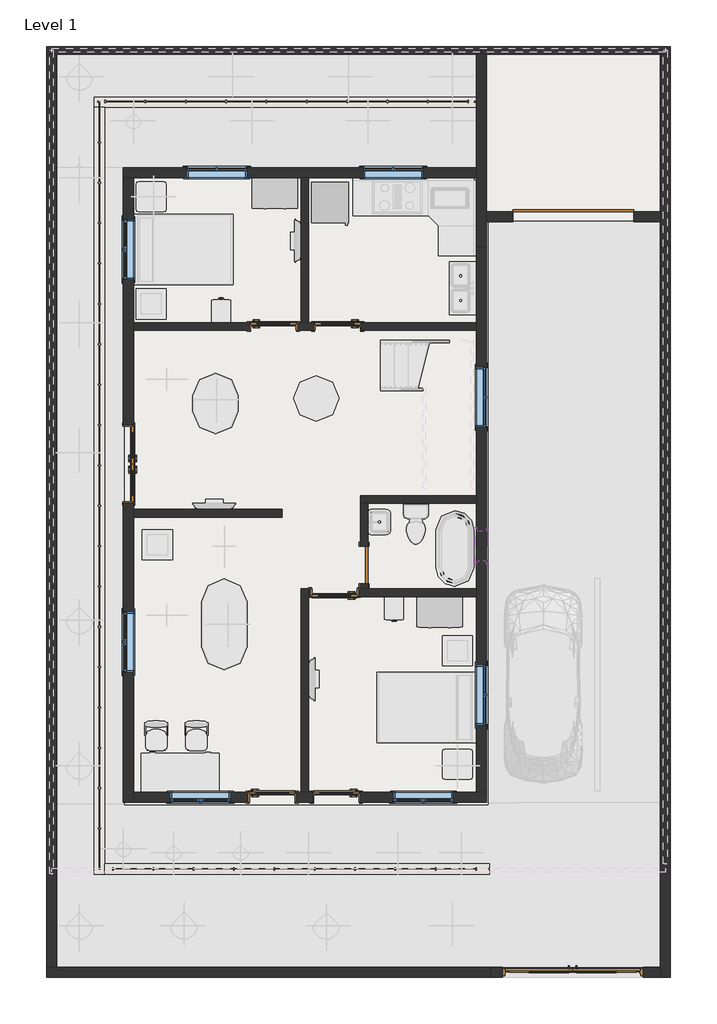
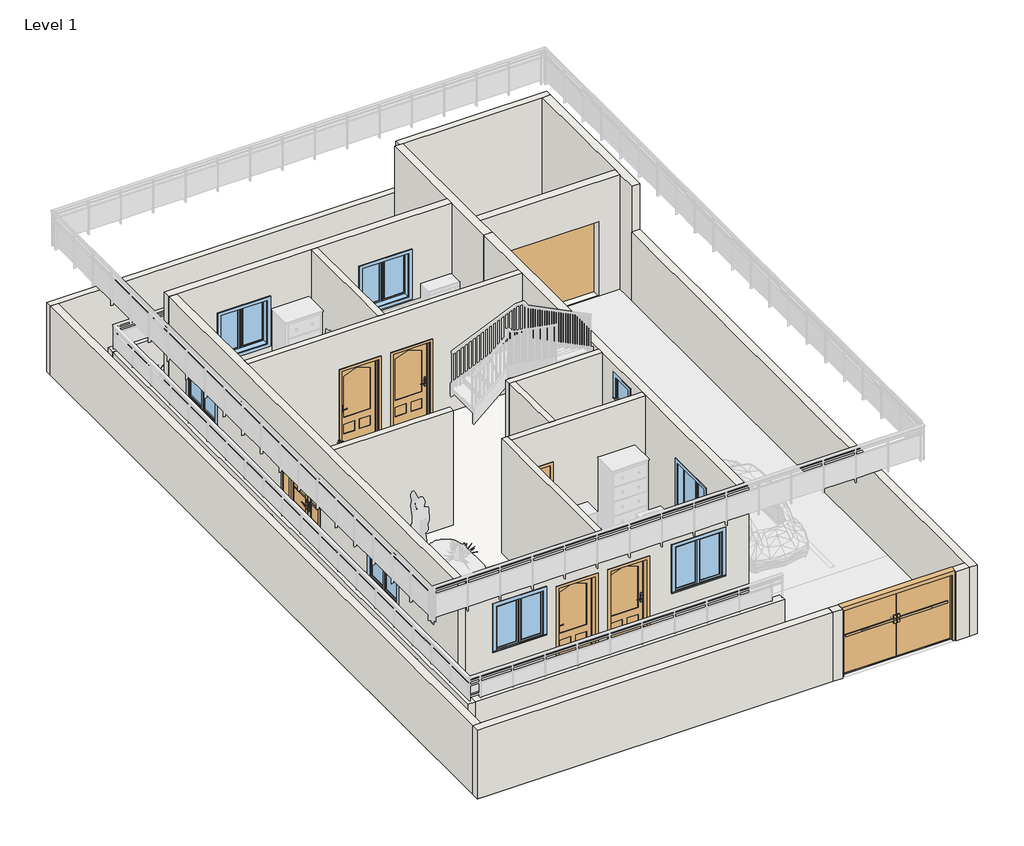
# One storey, part 1 of 5: 23 walls, 9 doors, 9 windows, 1 slab.
"""IFC4 building model written with IfcOpenShell, lengths in millimetres."""

from ifc_helpers import new_model, si_unit, frame, origin, origin_with_axes, place, context, project, spatial, polyline, outline, extrude, faceted_brep, transform, mapped, element, save
from components import door_62fd4200, door_5d363d20, door_808aeb8e, door_1768e003, door_exterior_double_door_exterior_double_ceddc7a2, door_b03bd389, door_be48eeb6, door_059fdd7e, window_0862ab64, window_e41d21a6

model = new_model("IFC4")

# Units and contexts
model_context = context("Model", 3, world=origin())
ifc_project = project(units=[si_unit("LENGTHUNIT", "METRE", prefix="MILLI")], contexts=[model_context])

# Site, building, storey
site = spatial("IfcSite", under=ifc_project)
building = spatial("IfcBuilding", under=site)
storey = spatial("IfcBuildingStorey", under=building, Name="Level 1", Elevation=0.0)

# Doors
placement = place(None, origin())
door_shape = door_62fd4200(model_context)
element("IfcDoor", 1, ObjectType="36\" x 80\"", at=placement, inside=storey, context=model_context, shape_type="MappedRepresentation", body=[
    mapped(door_shape, transform((-6591.1350785, -3422.7216995, 0.0), x_axis=(-1.0, 0.0, 0.0), y_axis=(0.0, -1.0, 0.0), z_axis=(0.0, 0.0, 1.0))),
])
door_2_shape = door_5d363d20(model_context)
element("IfcDoor", 2, ObjectType="36\" x 80\"", at=placement, inside=storey, context=model_context, shape_type="MappedRepresentation", body=[
    mapped(door_2_shape, transform((-6565.7350785, 6051.4783005, 0.0), x_axis=(-1.0, 0.0, 0.0), y_axis=(0.0, -1.0, 0.0), z_axis=(0.0, 0.0, 1.0))),
])
element("IfcDoor", 3, ObjectType="36\" x 80\"", at=placement, inside=storey, context=model_context, shape_type="MappedRepresentation", body=[
    mapped(door_2_shape, transform((-5333.8350785, 685.7283005, 0.0), x_axis=(1.0, 0.0, 0.0), y_axis=(0.0, 1.0, 0.0), z_axis=(0.0, 0.0, 1.0))),
])
door_3_shape = door_808aeb8e(model_context)
element("IfcDoor", 4, ObjectType="36\" x 80\"", at=placement, inside=storey, context=model_context, shape_type="MappedRepresentation", body=[
    mapped(door_3_shape, transform((-5270.3350785, 6051.4783005, 0.0), x_axis=(1.0, 0.0, 0.0), y_axis=(0.0, 1.0, 0.0), z_axis=(0.0, 0.0, 1.0))),
])
door_4_shape = door_1768e003(model_context)
element("IfcDoor", 5, ObjectType="36\" x 80\"", at=placement, inside=storey, context=model_context, shape_type="MappedRepresentation", body=[
    mapped(door_4_shape, transform((-5295.7350785, -3422.7216995, 0.0), x_axis=(1.0, 0.0, 0.0), y_axis=(0.0, 1.0, 0.0), z_axis=(0.0, 0.0, 1.0))),
])
door_exterior_double_door_exterior_double_shape = door_exterior_double_door_exterior_double_ceddc7a2(model_context)
element("IfcDoor", 6, ObjectType="Door-Exterior-Double : Door-Exterior-Double", at=placement, inside=storey, context=model_context, shape_type="MappedRepresentation", body=[
    mapped(door_exterior_double_door_exterior_double_shape, transform((-533.2350785, -6962.8466995, 0.0), x_axis=(1.0, 0.0, 0.0), y_axis=(0.0, 1.0, 0.0), z_axis=(0.0, 0.0, 1.0))),
])
door_5_shape = door_b03bd389(model_context)
element("IfcDoor", 7, ObjectType="Door-Exterior-Double-Full Glass-Wood_Clad : 60\" x 80\"", at=placement, inside=storey, context=model_context, shape_type="MappedRepresentation", body=[
    mapped(door_5_shape, transform((-9483.5600785, 3279.7033005, 0.0), x_axis=(0.0, -1.0, 0.0), y_axis=(1.0, 0.0, 0.0), z_axis=(0.0, 0.0, 1.0))),
])
door_6_shape = door_be48eeb6(model_context)
element("IfcDoor", 8, ObjectType="Door-Overhead-Sectional : 8' x 6'-6\"", at=placement, inside=storey, context=model_context, shape_type="MappedRepresentation", body=[
    mapped(door_6_shape, transform((-520.5350785, 8258.1033005, 0.0), x_axis=(-1.0, 0.0, 0.0), y_axis=(0.0, -1.0, 0.0), z_axis=(0.0, 0.0, 1.0))),
])
door_7_shape = door_059fdd7e(model_context)
element("IfcDoor", 9, ObjectType="Single-Flush : 30\" x 80\"", at=placement, inside=storey, context=model_context, shape_type="MappedRepresentation", body=[
    mapped(door_7_shape, transform((-4736.9350785, 1247.7033005, 0.0), x_axis=(0.0, -1.0, 0.0), y_axis=(1.0, 0.0, 0.0), z_axis=(0.0, 0.0, 1.0))),
])

# Slab
element("IfcSlab", 10, ObjectType="Generic - 12\"", at=placement, inside=storey, context=model_context, shape_type="SweptSolid", body=[
    extrude(outline(polyline([(-2273.1350785, 9248.7033005), (-2273.1350785, 11534.7033005), (1409.8649215, 11534.7033005), (1409.8649215, 8181.9033005), (-2247.7350785, 8181.9033005), (-2247.7350785, -3578.2966995), (-9562.9350785, -3578.2966995), (-9562.9350785, 9248.7033005), (-2273.1350785, 9248.7033005)])), frame((0.0, 0.0, -304.8), z_axis=(0.0, 0.0, 1.0), x_axis=(1.0, 0.0, 0.0)), (0.0, 0.0, 1.0), 304.8),
])

# Walls
element("IfcWall", 11, ObjectType="Generic - 2'", at=placement, inside=storey, context=model_context, shape_type="Brep", body=[
    faceted_brep([(-2476.3350785, 10671.1033005, 0.0), (-10172.5350785, 10671.1033005, 0.0), (-10172.5350785, 10671.1033005, 914.4), (-2476.3350785, 10671.1033005, 914.4), (-2476.3350785, 10467.9033005, 0.0), (-2476.3350785, 10467.9033005, 914.4), (-9969.3350785, 10467.9033005, 914.4), (-10172.5350785, 10467.9033005, 914.4), (-10172.5350785, 10467.9033005, 0.0), (-9969.3350785, 10467.9033005, 0.0)], [[[0, 1, 2, 3]], [[4, 5, 6, 7, 8, 9]], [[1, 0, 4, 9, 8]], [[3, 2, 7, 6, 5]], [[2, 1, 8, 7]], [[0, 3, 5, 4]]]),
])
element("IfcWall", 12, ObjectType="Generic - 2'", at=placement, inside=storey, context=model_context, shape_type="Brep", body=[
    faceted_brep([(-10172.5350785, 10467.9033005, 0.0), (-10172.5350785, -4975.2966995, 0.0), (-10172.5350785, -4975.2966995, 914.4), (-10172.5350785, 10467.9033005, 914.4), (-9969.3350785, 10467.9033005, 0.0), (-9969.3350785, 10467.9033005, 914.4), (-9969.3350785, -4772.0966995, 914.4), (-9969.3350785, -4975.2966995, 914.4), (-9969.3350785, -4975.2966995, 0.0), (-9969.3350785, -4772.0966995, 0.0)], [[[0, 1, 2, 3]], [[4, 5, 6, 7, 8, 9]], [[1, 0, 4, 9, 8]], [[3, 2, 7, 6, 5]], [[0, 3, 5, 4]], [[2, 1, 8, 7]]]),
])
element("IfcWall", 13, ObjectType="Generic - 2'", at=placement, inside=storey, context=model_context, shape_type="SweptSolid", body=[
    extrude(outline(polyline([(-2209.6350785, -4975.2966995), (-9969.3350785, -4975.2966995), (-9969.3350785, -4772.0966995), (-2209.6350785, -4772.0966995), (-2209.6350785, -4975.2966995)])), origin_with_axes(), (0.0, 0.0, 1.0), 914.4),
])
element("IfcWall", 14, ObjectType="Generic - 8\"", at=placement, inside=storey, context=model_context, shape_type="Brep", body=[
    faceted_brep([(-9385.1350785, 9045.5033005, 0.0), (-9385.1350785, 9045.5033005, 3048.0), (-9385.1350785, 6124.5033005, 3048.0), (-9385.1350785, 5972.1033005, 3048.0), (-9385.1350785, 2365.3033005, 3048.0), (-9385.1350785, 2212.9033005, 3048.0), (-9385.1350785, -3324.2966995, 3048.0), (-9385.1350785, -3527.4966995, 3048.0), (-9385.1350785, -3527.4966995, 0.0), (-9385.1350785, -3324.2966995, 0.0), (-9385.1350785, 2212.9033005, 0.0), (-9385.1350785, 2365.3033005, 0.0), (-9385.1350785, 2492.3033005, 0.0), (-9385.1350785, 2492.3033005, 2057.4), (-9385.1350785, 4067.1033005, 2057.4), (-9385.1350785, 4067.1033005, 0.0), (-9385.1350785, 5972.1033005, 0.0), (-9385.1350785, 6124.5033005, 0.0), (-9385.1350785, 8207.3033005, 2133.6), (-9385.1350785, 8207.3033005, 914.4), (-9385.1350785, 6988.1033005, 914.4), (-9385.1350785, 6988.1033005, 2133.6), (-9385.1350785, 307.9033005, 2133.6), (-9385.1350785, 307.9033005, 914.4), (-9385.1350785, -911.2966995, 914.4), (-9385.1350785, -911.2966995, 2133.6), (-9588.3350785, 9045.5033005, 3048.0), (-9588.3350785, 9045.5033005, 0.0), (-9588.3350785, 4067.1033005, 0.0), (-9588.3350785, 4067.1033005, 2057.4), (-9588.3350785, 2492.3033005, 2057.4), (-9588.3350785, 2492.3033005, 0.0), (-9588.3350785, -3527.4966995, 0.0), (-9588.3350785, -3527.4966995, 3048.0), (-9588.3350785, 8207.3033005, 2133.6), (-9588.3350785, 6988.1033005, 2133.6), (-9588.3350785, 6988.1033005, 914.4), (-9588.3350785, 8207.3033005, 914.4), (-9588.3350785, 307.9033005, 2133.6), (-9588.3350785, -911.2966995, 2133.6), (-9588.3350785, -911.2966995, 914.4), (-9588.3350785, 307.9033005, 914.4)], [[[0, 1, 2, 3, 4, 5, 6, 7, 8, 9, 10, 11, 12, 13, 14, 15, 16, 17], [18, 19, 20, 21], [22, 23, 24, 25]], [[26, 27, 28, 29, 30, 31, 32, 33], [34, 35, 36, 37], [38, 39, 40, 41]], [[27, 0, 17, 16, 15, 28]], [[8, 32, 31, 12, 11, 10, 9]], [[1, 0, 27, 26]], [[8, 7, 33, 32]], [[19, 18, 34, 37]], [[20, 19, 37, 36]], [[21, 20, 36, 35]], [[18, 21, 35, 34]], [[23, 22, 38, 41]], [[24, 23, 41, 40]], [[25, 24, 40, 39]], [[22, 25, 39, 38]], [[7, 6, 5, 4, 3, 2, 1, 26, 33]], [[30, 13, 12, 31]], [[13, 30, 29, 14]], [[14, 29, 28, 15]]]),
])
element("IfcWall", 15, ObjectType="Generic - 8\"", at=placement, inside=storey, context=model_context, shape_type="Brep", body=[
    faceted_brep([(-9588.3350785, 9045.5033005, 0.0), (-9385.1350785, 9045.5033005, 0.0), (-6006.9350785, 9045.5033005, 0.0), (-5854.5350785, 9045.5033005, 0.0), (-2476.3350785, 9045.5033005, 0.0), (-2476.3350785, 9045.5033005, 3048.0), (-5854.5350785, 9045.5033005, 3048.0), (-6006.9350785, 9045.5033005, 3048.0), (-9385.1350785, 9045.5033005, 3048.0), (-9588.3350785, 9045.5033005, 3048.0), (-7099.1350785, 9045.5033005, 2133.6), (-7099.1350785, 9045.5033005, 914.4), (-8318.3350785, 9045.5033005, 914.4), (-8318.3350785, 9045.5033005, 2133.6), (-3543.1350785, 9045.5033005, 2133.6), (-3543.1350785, 9045.5033005, 914.4), (-4762.3350785, 9045.5033005, 914.4), (-4762.3350785, 9045.5033005, 2133.6), (-9588.3350785, 9248.7033005, 0.0), (-9588.3350785, 9248.7033005, 3048.0), (-2476.3350785, 9248.7033005, 3048.0), (-2476.3350785, 9248.7033005, 0.0), (-7099.1350785, 9248.7033005, 2133.6), (-8318.3350785, 9248.7033005, 2133.6), (-8318.3350785, 9248.7033005, 914.4), (-7099.1350785, 9248.7033005, 914.4), (-3543.1350785, 9248.7033005, 2133.6), (-4762.3350785, 9248.7033005, 2133.6), (-4762.3350785, 9248.7033005, 914.4), (-3543.1350785, 9248.7033005, 914.4)], [[[0, 1, 2, 3, 4, 5, 6, 7, 8, 9], [10, 11, 12, 13], [14, 15, 16, 17]], [[18, 19, 20, 21], [22, 23, 24, 25], [26, 27, 28, 29]], [[4, 3, 2, 1, 0, 18, 21]], [[0, 9, 19, 18]], [[5, 4, 21, 20]], [[11, 10, 22, 25]], [[12, 11, 25, 24]], [[13, 12, 24, 23]], [[10, 13, 23, 22]], [[15, 14, 26, 29]], [[16, 15, 29, 28]], [[17, 16, 28, 27]], [[14, 17, 27, 26]], [[9, 8, 7, 6, 5, 20, 19]]]),
])
element("IfcWall", 16, ObjectType="Generic - 8\"", at=placement, inside=storey, context=model_context, shape_type="Brep", body=[
    faceted_brep([(-2273.1350785, -3324.2966995, 0.0), (-2273.1350785, 7648.5033005, 0.0), (-2273.1350785, 7648.5033005, 3048.0), (-2273.1350785, -3324.2966995, 3048.0), (-2273.1350785, -1978.0966995, 2133.6), (-2273.1350785, -758.8966995, 2133.6), (-2273.1350785, -758.8966995, 914.4), (-2273.1350785, -1978.0966995, 914.4), (-2273.1350785, 4016.3033005, 2133.6), (-2273.1350785, 5235.5033005, 2133.6), (-2273.1350785, 5235.5033005, 914.4), (-2273.1350785, 4016.3033005, 914.4), (-2273.1350785, 1933.5033005, 2768.6), (-2273.1350785, 1933.5033005, 2159.0), (-2273.1350785, 1323.9033005, 2159.0), (-2273.1350785, 1323.9033005, 2768.6), (-2476.3350785, -3324.2966995, 0.0), (-2476.3350785, -3324.2966995, 3048.0), (-2476.3350785, 612.7033005, 3048.0), (-2476.3350785, 765.1033005, 3048.0), (-2476.3350785, 2492.3033005, 3048.0), (-2476.3350785, 2644.7033005, 3048.0), (-2476.3350785, 5972.1033005, 3048.0), (-2476.3350785, 6124.5033005, 3048.0), (-2476.3350785, 7648.5033005, 3048.0), (-2476.3350785, 7648.5033005, 0.0), (-2476.3350785, 6124.5033005, 0.0), (-2476.3350785, 5972.1033005, 0.0), (-2476.3350785, 2644.7033005, 0.0), (-2476.3350785, 2492.3033005, 0.0), (-2476.3350785, 765.1033005, 0.0), (-2476.3350785, 612.7033005, 0.0), (-2476.3350785, -1978.0966995, 2133.6), (-2476.3350785, -1978.0966995, 914.4), (-2476.3350785, -758.8966995, 914.4), (-2476.3350785, -758.8966995, 2133.6), (-2476.3350785, 4016.3033005, 2133.6), (-2476.3350785, 4016.3033005, 914.4), (-2476.3350785, 5235.5033005, 914.4), (-2476.3350785, 5235.5033005, 2133.6), (-2476.3350785, 1933.5033005, 2768.6), (-2476.3350785, 1323.9033005, 2768.6), (-2476.3350785, 1323.9033005, 2159.0), (-2476.3350785, 1933.5033005, 2159.0)], [[[0, 1, 2, 3], [4, 5, 6, 7], [8, 9, 10, 11], [12, 13, 14, 15]], [[16, 17, 18, 19, 20, 21, 22, 23, 24, 25, 26, 27, 28, 29, 30, 31], [32, 33, 34, 35], [36, 37, 38, 39], [40, 41, 42, 43]], [[1, 0, 16, 31, 30, 29, 28, 27, 26, 25]], [[2, 1, 25, 24]], [[0, 3, 17, 16]], [[33, 32, 4, 7]], [[34, 33, 7, 6]], [[35, 34, 6, 5]], [[32, 35, 5, 4]], [[37, 36, 8, 11]], [[38, 37, 11, 10]], [[39, 38, 10, 9]], [[36, 39, 9, 8]], [[13, 12, 40, 43]], [[14, 13, 43, 42]], [[15, 14, 42, 41]], [[12, 15, 41, 40]], [[3, 2, 24, 23, 22, 21, 20, 19, 18, 17]]]),
])
element("IfcWall", 17, ObjectType="Generic - 8\"", at=placement, inside=storey, context=model_context, shape_type="Brep", body=[
    faceted_brep([(-9385.1350785, -3527.4966995, 3048.0), (-9385.1350785, -3527.4966995, 0.0), (-7073.7350785, -3527.4966995, 0.0), (-7073.7350785, -3527.4966995, 2057.4), (-6108.5350785, -3527.4966995, 2057.4), (-6108.5350785, -3527.4966995, 0.0), (-5778.3350785, -3527.4966995, 0.0), (-5778.3350785, -3527.4966995, 2057.4), (-4813.1350785, -3527.4966995, 2057.4), (-4813.1350785, -3527.4966995, 0.0), (-2273.1350785, -3527.4966995, 0.0), (-2273.1350785, -3527.4966995, 3048.0), (-8648.5350785, -3527.4966995, 2133.6), (-7429.3350785, -3527.4966995, 2133.6), (-7429.3350785, -3527.4966995, 914.4), (-8648.5350785, -3527.4966995, 914.4), (-4152.7350785, -3527.4966995, 2133.6), (-2933.5350785, -3527.4966995, 2133.6), (-2933.5350785, -3527.4966995, 914.4), (-4152.7350785, -3527.4966995, 914.4), (-9385.1350785, -3324.2966995, 0.0), (-9385.1350785, -3324.2966995, 3048.0), (-6006.9350785, -3324.2966995, 3048.0), (-5854.5350785, -3324.2966995, 3048.0), (-2476.3350785, -3324.2966995, 3048.0), (-2273.1350785, -3324.2966995, 3048.0), (-2273.1350785, -3324.2966995, 0.0), (-2476.3350785, -3324.2966995, 0.0), (-4813.1350785, -3324.2966995, 0.0), (-4813.1350785, -3324.2966995, 2057.4), (-5778.3350785, -3324.2966995, 2057.4), (-5778.3350785, -3324.2966995, 0.0), (-5854.5350785, -3324.2966995, 0.0), (-6006.9350785, -3324.2966995, 0.0), (-6108.5350785, -3324.2966995, 0.0), (-6108.5350785, -3324.2966995, 2057.4), (-7073.7350785, -3324.2966995, 2057.4), (-7073.7350785, -3324.2966995, 0.0), (-8648.5350785, -3324.2966995, 2133.6), (-8648.5350785, -3324.2966995, 914.4), (-7429.3350785, -3324.2966995, 914.4), (-7429.3350785, -3324.2966995, 2133.6), (-4152.7350785, -3324.2966995, 2133.6), (-4152.7350785, -3324.2966995, 914.4), (-2933.5350785, -3324.2966995, 914.4), (-2933.5350785, -3324.2966995, 2133.6)], [[[0, 1, 2, 3, 4, 5, 6, 7, 8, 9, 10, 11], [12, 13, 14, 15], [16, 17, 18, 19]], [[20, 21, 22, 23, 24, 25, 26, 27, 28, 29, 30, 31, 32, 33, 34, 35, 36, 37], [38, 39, 40, 41], [42, 43, 44, 45]], [[1, 20, 37, 2]], [[26, 10, 9, 28, 27]], [[5, 34, 33, 32, 31, 6]], [[1, 0, 21, 20]], [[11, 10, 26, 25]], [[36, 3, 2, 37]], [[3, 36, 35, 4]], [[4, 35, 34, 5]], [[39, 38, 12, 15]], [[40, 39, 15, 14]], [[41, 40, 14, 13]], [[38, 41, 13, 12]], [[43, 42, 16, 19]], [[44, 43, 19, 18]], [[45, 44, 18, 17]], [[42, 45, 17, 16]], [[0, 11, 25, 24, 23, 22, 21]], [[8, 29, 28, 9]], [[29, 8, 7, 30]], [[30, 7, 6, 31]]]),
])
element("IfcWall", 18, ObjectType="Generic - 8\"", at=placement, inside=storey, context=model_context, shape_type="Brep", body=[
    faceted_brep([(-2273.1350785, 7648.5033005, 0.0), (-2273.1350785, 8156.5033005, 0.0), (-2273.1350785, 8359.7033005, 0.0), (-2273.1350785, 11534.7033005, 0.0), (-2273.1350785, 11534.7033005, 3048.0), (-2273.1350785, 8359.7033005, 3048.0), (-2273.1350785, 8156.5033005, 3048.0), (-2273.1350785, 7648.5033005, 3048.0), (-2476.3350785, 7648.5033005, 0.0), (-2476.3350785, 7648.5033005, 3048.0), (-2476.3350785, 9045.5033005, 3048.0), (-2476.3350785, 9248.7033005, 3048.0), (-2476.3350785, 11534.7033005, 3048.0), (-2476.3350785, 11534.7033005, 0.0), (-2476.3350785, 10671.1033005, 0.0), (-2476.3350785, 10467.9033005, 0.0), (-2476.3350785, 9248.7033005, 0.0), (-2476.3350785, 9045.5033005, 0.0), (-2362.0350785, 11534.7033005, 0.0), (-2362.0350785, 11534.7033005, 3048.0)], [[[0, 1, 2, 3, 4, 5, 6, 7]], [[8, 9, 10, 11, 12, 13, 14, 15, 16, 17]], [[3, 2, 1, 0, 8, 17, 16, 15, 14, 13, 18]], [[0, 7, 9, 8]], [[4, 3, 18, 13, 12, 19]], [[7, 6, 5, 4, 19, 12, 11, 10, 9]]]),
])
element("IfcWall", 19, ObjectType="Generic - 8\"", at=placement, inside=storey, context=model_context, shape_type="SweptSolid", body=[
    extrude(outline(polyline([(0.0, 1232.0649215), (3048.0, 1232.0649215), (3048.0, -2273.1350785), (0.0, -2273.1350785), (0.0, -1739.7350785), (1981.2, -1739.7350785), (1981.2, 698.6649215), (0.0, 698.6649215), (0.0, 1232.0649215)])), frame((0.0, 8156.5033005, 0.0), z_axis=(0.0, 1.0, 0.0), x_axis=(0.0, 0.0, 1.0)), (0.0, 0.0, 1.0), 203.2),
])
element("IfcWall", 20, ObjectType="INNER 6\"", at=placement, inside=storey, context=model_context, shape_type="Brep", body=[
    faceted_brep([(-11137.7350785, 11534.7033005, 0.0), (-10934.5350785, 11534.7033005, 0.0), (-2387.4350785, 11534.7033005, 0.0), (-2387.4350785, 11534.7033005, 1828.8), (-10934.5350785, 11534.7033005, 1828.8), (-11137.7350785, 11534.7033005, 1828.8), (-11137.7350785, 11687.1033005, 0.0), (-11137.7350785, 11687.1033005, 1828.8), (-2387.4350785, 11687.1033005, 1828.8), (-2387.4350785, 11687.1033005, 0.0)], [[[0, 1, 2, 3, 4, 5]], [[6, 7, 8, 9]], [[2, 1, 0, 6, 9]], [[3, 2, 9, 8]], [[5, 4, 3, 8, 7]], [[0, 5, 7, 6]]]),
])
element("IfcWall", 21, ObjectType="INNER 6\"", at=placement, inside=storey, context=model_context, shape_type="SweptSolid", body=[
    extrude(outline(polyline([(-6006.9350785, 6124.5033005), (-6006.9350785, 9045.5033005), (-5854.5350785, 9045.5033005), (-5854.5350785, 6124.5033005), (-6006.9350785, 6124.5033005)])), origin_with_axes(), (0.0, 0.0, 1.0), 3048.0),
])
element("IfcWall", 22, ObjectType="INNER 6\"", at=placement, inside=storey, context=model_context, shape_type="Brep", body=[
    faceted_brep([(-9385.1350785, 6124.5033005, 0.0), (-9385.1350785, 6124.5033005, 3048.0), (-6006.9350785, 6124.5033005, 3048.0), (-5854.5350785, 6124.5033005, 3048.0), (-2476.3350785, 6124.5033005, 3048.0), (-2476.3350785, 6124.5033005, 0.0), (-4787.7350785, 6124.5033005, 0.0), (-4787.7350785, 6124.5033005, 2057.4), (-5752.9350785, 6124.5033005, 2057.4), (-5752.9350785, 6124.5033005, 0.0), (-5854.5350785, 6124.5033005, 0.0), (-6006.9350785, 6124.5033005, 0.0), (-6083.1350785, 6124.5033005, 0.0), (-6083.1350785, 6124.5033005, 2057.4), (-7048.3350785, 6124.5033005, 2057.4), (-7048.3350785, 6124.5033005, 0.0), (-9385.1350785, 5972.1033005, 3048.0), (-9385.1350785, 5972.1033005, 0.0), (-7048.3350785, 5972.1033005, 0.0), (-7048.3350785, 5972.1033005, 2057.4), (-6083.1350785, 5972.1033005, 2057.4), (-6083.1350785, 5972.1033005, 0.0), (-5752.9350785, 5972.1033005, 0.0), (-5752.9350785, 5972.1033005, 2057.4), (-4787.7350785, 5972.1033005, 2057.4), (-4787.7350785, 5972.1033005, 0.0), (-2476.3350785, 5972.1033005, 0.0), (-2476.3350785, 5972.1033005, 3048.0)], [[[0, 1, 2, 3, 4, 5, 6, 7, 8, 9, 10, 11, 12, 13, 14, 15]], [[16, 17, 18, 19, 20, 21, 22, 23, 24, 25, 26, 27]], [[5, 26, 25, 6]], [[17, 0, 15, 18]], [[21, 12, 11, 10, 9, 22]], [[1, 0, 17, 16]], [[5, 4, 27, 26]], [[14, 19, 18, 15]], [[19, 14, 13, 20]], [[20, 13, 12, 21]], [[24, 7, 6, 25]], [[7, 24, 23, 8]], [[8, 23, 22, 9]], [[4, 3, 2, 1, 16, 27]]]),
])
element("IfcWall", 23, ObjectType="INNER 6\"", at=placement, inside=storey, context=model_context, shape_type="SweptSolid", body=[
    extrude(outline(polyline([(-6387.9350785, 2212.9033005), (-9385.1350785, 2212.9033005), (-9385.1350785, 2365.3033005), (-6387.9350785, 2365.3033005), (-6387.9350785, 2212.9033005)])), origin_with_axes(), (0.0, 0.0, 1.0), 3048.0),
])
element("IfcWall", 24, ObjectType="INNER 6\"", at=placement, inside=storey, context=model_context, shape_type="Brep", body=[
    faceted_brep([(-5854.5350785, -3324.2966995, 0.0), (-5854.5350785, 612.7033005, 0.0), (-5854.5350785, 765.1033005, 0.0), (-5854.5350785, 765.1033005, 3048.0), (-5854.5350785, 612.7033005, 3048.0), (-5854.5350785, -3324.2966995, 3048.0), (-6006.9350785, -3324.2966995, 0.0), (-6006.9350785, -3324.2966995, 3048.0), (-6006.9350785, 765.1033005, 3048.0), (-6006.9350785, 765.1033005, 0.0)], [[[0, 1, 2, 3, 4, 5]], [[6, 7, 8, 9]], [[2, 1, 0, 6, 9]], [[0, 5, 7, 6]], [[3, 2, 9, 8]], [[5, 4, 3, 8, 7]]]),
])
element("IfcWall", 25, ObjectType="INNER 6\"", at=placement, inside=storey, context=model_context, shape_type="Brep", body=[
    faceted_brep([(-2476.3350785, 765.1033005, 3048.0), (-2476.3350785, 765.1033005, 0.0), (-4660.7350785, 765.1033005, 0.0), (-4813.1350785, 765.1033005, 0.0), (-4851.2350785, 765.1033005, 0.0), (-4851.2350785, 765.1033005, 2057.4), (-5816.4350785, 765.1033005, 2057.4), (-5816.4350785, 765.1033005, 0.0), (-5854.5350785, 765.1033005, 0.0), (-5854.5350785, 765.1033005, 3048.0), (-4813.1350785, 765.1033005, 3048.0), (-4660.7350785, 765.1033005, 3048.0), (-2476.3350785, 612.7033005, 0.0), (-2476.3350785, 612.7033005, 3048.0), (-5854.5350785, 612.7033005, 3048.0), (-5854.5350785, 612.7033005, 0.0), (-5816.4350785, 612.7033005, 0.0), (-5816.4350785, 612.7033005, 2057.4), (-4851.2350785, 612.7033005, 2057.4), (-4851.2350785, 612.7033005, 0.0)], [[[0, 1, 2, 3, 4, 5, 6, 7, 8, 9, 10, 11]], [[12, 13, 14, 15, 16, 17, 18, 19]], [[1, 12, 19, 4, 3, 2]], [[15, 8, 7, 16]], [[1, 0, 13, 12]], [[9, 8, 15, 14]], [[18, 5, 4, 19]], [[5, 18, 17, 6]], [[6, 17, 16, 7]], [[0, 11, 10, 9, 14, 13]]]),
])
element("IfcWall", 26, ObjectType="INNER 6\"", at=placement, inside=storey, context=model_context, shape_type="SweptSolid", body=[
    extrude(outline(polyline([(866.7033005, 2032.0), (866.7033005, 0.0), (765.1033005, 0.0), (765.1033005, 3048.0), (2492.3033005, 3048.0), (2492.3033005, 0.0), (1628.7033005, 0.0), (1628.7033005, 2032.0), (866.7033005, 2032.0)])), frame((-4813.1350785, 0.0, 0.0), z_axis=(1.0, 0.0, 0.0), x_axis=(0.0, 1.0, 0.0)), (0.0, 0.0, 1.0), 152.4),
])
element("IfcWall", 27, ObjectType="INNER 6\"", at=placement, inside=storey, context=model_context, shape_type="Brep", body=[
    faceted_brep([(-4813.1350785, 2492.3033005, 0.0), (-4660.7350785, 2492.3033005, 0.0), (-2476.3350785, 2492.3033005, 0.0), (-2476.3350785, 2492.3033005, 3048.0), (-4660.7350785, 2492.3033005, 3048.0), (-4813.1350785, 2492.3033005, 3048.0), (-4813.1350785, 2644.7033005, 0.0), (-4813.1350785, 2644.7033005, 3048.0), (-2476.3350785, 2644.7033005, 3048.0), (-2476.3350785, 2644.7033005, 0.0)], [[[0, 1, 2, 3, 4, 5]], [[6, 7, 8, 9]], [[2, 1, 0, 6, 9]], [[3, 2, 9, 8]], [[0, 5, 7, 6]], [[5, 4, 3, 8, 7]]]),
])
element("IfcWall", 28, ObjectType="INNER 6\" 2", at=placement, inside=storey, context=model_context, shape_type="Brep", body=[
    faceted_brep([(-2362.0350785, 11534.7033005, 0.0), (-2273.1350785, 11534.7033005, 0.0), (1232.0649215, 11534.7033005, 0.0), (1435.2649215, 11534.7033005, 0.0), (1435.2649215, 11534.7033005, 3048.0), (1232.0649215, 11534.7033005, 3048.0), (-2273.1350785, 11534.7033005, 3048.0), (-2362.0350785, 11534.7033005, 3048.0), (-2362.0350785, 11687.1033005, 0.0), (-2362.0350785, 11687.1033005, 3048.0), (1435.2649215, 11687.1033005, 3048.0), (1435.2649215, 11687.1033005, 0.0)], [[[0, 1, 2, 3, 4, 5, 6, 7]], [[8, 9, 10, 11]], [[3, 2, 1, 0, 8, 11]], [[0, 7, 9, 8]], [[4, 3, 11, 10]], [[7, 6, 5, 4, 10, 9]]]),
])
element("IfcWall", 29, ObjectType="OUTER WALL 6'", at=placement, inside=storey, context=model_context, shape_type="SweptSolid", body=[
    extrude(outline(polyline([(-10934.5350785, 11534.7033005), (-10934.5350785, -6854.8966995), (-11137.7350785, -6854.8966995), (-11137.7350785, 11534.7033005), (-10934.5350785, 11534.7033005)])), origin_with_axes(), (0.0, 0.0, 1.0), 1828.8),
])
element("IfcWall", 30, ObjectType="OUTER WALL 6'", at=placement, inside=storey, context=model_context, shape_type="Brep", body=[
    faceted_brep([(-2196.9350785, -6854.8966995, 0.0), (-10934.5350785, -6854.8966995, 0.0), (-11137.7350785, -6854.8966995, 0.0), (-11137.7350785, -6854.8966995, 1828.8), (-10934.5350785, -6854.8966995, 1828.8), (-2196.9350785, -6854.8966995, 1828.8), (-2196.9350785, -7058.0966995, 0.0), (-2196.9350785, -7058.0966995, 1828.8), (-11137.7350785, -7058.0966995, 1828.8), (-11137.7350785, -7058.0966995, 0.0)], [[[0, 1, 2, 3, 4, 5]], [[6, 7, 8, 9]], [[2, 1, 0, 6, 9]], [[5, 4, 3, 8, 7]], [[0, 5, 7, 6]], [[3, 2, 9, 8]]]),
])
element("IfcWall", 31, ObjectType="OUTER WALL 6'", at=placement, inside=storey, context=model_context, shape_type="Brep", body=[
    faceted_brep([(1232.0649215, 7648.5033005, 0.0), (1232.0649215, -6854.8966995, 0.0), (1232.0649215, -7058.0966995, 0.0), (1232.0649215, -7058.0966995, 1828.8), (1232.0649215, -6854.8966995, 1828.8), (1232.0649215, 7648.5033005, 1828.8), (1435.2649215, 7648.5033005, 0.0), (1435.2649215, 7648.5033005, 1828.8), (1435.2649215, -7058.0966995, 1828.8), (1435.2649215, -7058.0966995, 0.0)], [[[0, 1, 2, 3, 4, 5]], [[6, 7, 8, 9]], [[2, 1, 0, 6, 9]], [[3, 2, 9, 8]], [[5, 4, 3, 8, 7]], [[0, 5, 7, 6]]]),
])
element("IfcWall", 32, ObjectType="OUTER WALL 6'", at=placement, inside=storey, context=model_context, shape_type="SweptSolid", body=[
    extrude(outline(polyline([(1232.0649215, -6854.8966995), (1232.0649215, -7058.0966995), (889.1649215, -7058.0966995), (889.1649215, -6854.8966995), (1232.0649215, -6854.8966995)])), origin_with_axes(), (0.0, 0.0, 1.0), 1828.8),
    extrude(outline(polyline([(-2196.9350785, -7058.0966995), (-2196.9350785, -6854.8966995), (-1955.6350785, -6854.8966995), (-1955.6350785, -7058.0966995), (-2196.9350785, -7058.0966995)])), origin_with_axes(), (0.0, 0.0, 1.0), 1828.8),
])
element("IfcWall", 33, ObjectType="OUTER WALL 6' 2", at=placement, inside=storey, context=model_context, shape_type="Brep", body=[
    faceted_brep([(1232.0649215, 11534.7033005, 0.0), (1232.0649215, 8359.7033005, 0.0), (1232.0649215, 8156.5033005, 0.0), (1232.0649215, 7648.5033005, 0.0), (1232.0649215, 7648.5033005, 3048.0), (1232.0649215, 8156.5033005, 3048.0), (1232.0649215, 8359.7033005, 3048.0), (1232.0649215, 11534.7033005, 3048.0), (1435.2649215, 11534.7033005, 0.0), (1435.2649215, 11534.7033005, 3048.0), (1435.2649215, 7648.5033005, 3048.0), (1435.2649215, 7648.5033005, 0.0)], [[[0, 1, 2, 3, 4, 5, 6, 7]], [[8, 9, 10, 11]], [[3, 2, 1, 0, 8, 11]], [[4, 3, 11, 10]], [[0, 7, 9, 8]], [[7, 6, 5, 4, 10, 9]]]),
])

# Windows
window_shape = window_0862ab64(model_context)
element("IfcWindow", 34, ObjectType="Casement Dbl with Trim : 48\" x 48\"", at=placement, inside=storey, context=model_context, shape_type="MappedRepresentation", body=[
    mapped(window_shape, transform((-7708.7350785, 9128.0533005, 0.0), x_axis=(1.0, 0.0, 0.0), y_axis=(0.0, 1.0, 0.0), z_axis=(0.0, 0.0, 1.0))),
])
element("IfcWindow", 35, ObjectType="Casement Dbl with Trim : 48\" x 48\"", at=placement, inside=storey, context=model_context, shape_type="MappedRepresentation", body=[
    mapped(window_shape, transform((-4152.7350785, 9128.0533005, 0.0), x_axis=(1.0, 0.0, 0.0), y_axis=(0.0, 1.0, 0.0), z_axis=(0.0, 0.0, 1.0))),
])
element("IfcWindow", 36, ObjectType="Casement Dbl with Trim : 48\" x 48\"", at=placement, inside=storey, context=model_context, shape_type="MappedRepresentation", body=[
    mapped(window_shape, transform((-9467.6850785, 7597.7033005, 0.0), x_axis=(0.0, 1.0, 0.0), y_axis=(-1.0, 0.0, 0.0), z_axis=(0.0, 0.0, 1.0))),
])
element("IfcWindow", 37, ObjectType="Casement Dbl with Trim : 48\" x 48\"", at=placement, inside=storey, context=model_context, shape_type="MappedRepresentation", body=[
    mapped(window_shape, transform((-8038.9350785, -3406.8466995, 0.0), x_axis=(-1.0, 0.0, 0.0), y_axis=(0.0, -1.0, 0.0), z_axis=(0.0, 0.0, 1.0))),
])
element("IfcWindow", 38, ObjectType="Casement Dbl with Trim : 48\" x 48\"", at=placement, inside=storey, context=model_context, shape_type="MappedRepresentation", body=[
    mapped(window_shape, transform((-9467.6850785, -301.6966995, 0.0), x_axis=(0.0, 1.0, 0.0), y_axis=(-1.0, 0.0, 0.0), z_axis=(0.0, 0.0, 1.0))),
])
element("IfcWindow", 39, ObjectType="Casement Dbl with Trim : 48\" x 48\"", at=placement, inside=storey, context=model_context, shape_type="MappedRepresentation", body=[
    mapped(window_shape, transform((-3543.1350785, -3406.8466995, 0.0), x_axis=(-1.0, 0.0, 0.0), y_axis=(0.0, -1.0, 0.0), z_axis=(0.0, 0.0, 1.0))),
])
element("IfcWindow", 40, ObjectType="Casement Dbl with Trim : 48\" x 48\"", at=placement, inside=storey, context=model_context, shape_type="MappedRepresentation", body=[
    mapped(window_shape, transform((-2393.7850785, -1368.4966995, 0.0), x_axis=(0.0, -1.0, 0.0), y_axis=(1.0, 0.0, 0.0), z_axis=(0.0, 0.0, 1.0))),
])
element("IfcWindow", 41, ObjectType="Casement Dbl with Trim : 48\" x 48\"", at=placement, inside=storey, context=model_context, shape_type="MappedRepresentation", body=[
    mapped(window_shape, transform((-2393.7850785, 4625.9033005, 0.0), x_axis=(0.0, -1.0, 0.0), y_axis=(1.0, 0.0, 0.0), z_axis=(0.0, 0.0, 1.0))),
])
window_2_shape = window_e41d21a6(model_context)
element("IfcWindow", 42, ObjectType="Transom with Trim : 24\" x 24\"", at=placement, inside=storey, context=model_context, shape_type="MappedRepresentation", body=[
    mapped(window_2_shape, transform((-2374.7350785, 1666.8033005, 0.0), x_axis=(0.0, 1.0, 0.0), y_axis=(-1.0, 0.0, 0.0), z_axis=(0.0, 0.0, 1.0))),
])

save(model, "model.ifc")

# Revit data of these elements
# Type "36\" x 80\""
#   Type Mark = "15"
#   Assembly Code = "B2030100"
#   Analytic Construction = "French door, wood frame with single glass"
#   Threshold Offset [instance default] = 0' - 0 1/2"
#   Thickness = 0' - 1 3/8"
#   Thermal Resistance (R) = 1.0696 (h·ft²·°F)/BTU
#   Swing Angle [instance default] = 90.00°
#   Stiles = 0' - 4 3/4"
#   Rough Width = 3' - 2"
#   Rough Height = 6' - 9"
#   Radius = 1' - 8.05625"
#   Lock Rail = 0' - 7 1/8"
#   Height = 6' - 8"
#   Width = 3' - 0"
#   Heat Transfer Coefficient (U) = 0.9350 BTU/(h·ft²·°F)
#   Door Offset [instance default] = 0' - 0"
#   Bottom Rail = 0' - 9 1/2"
#   Threshold [instance default] = yes
#   Function = 1
#   Exterior Trim [instance default] = yes
#   Trim Material = Cherry
#   Threshold Material = Cherry
#   Panel Material = Cherry
#   Glazing = Glass
#   Frame Material = Cherry
#   Door Handle Material = Aluminum
#   Visual Light Transmittance = 0
#   Solar Heat Gain Coefficient = 0
#   Wall Closure = (empty or 0)
#   Construction Type = (empty or 0)
# Type "Door-Exterior-Double : Door-Exterior-Double"
#   Type Mark = "19"
#   Assembly Code = "B2030200"
#   Analytic Construction = "Metal"
#   Threshold Length [instance default] = 9' - 4"
#   Threshold Offset [instance default] = 0' - 0 1/2"
#   Thickness = 0' - 1 3/4"
#   Thermal Resistance (R) = 1.5338 (h·ft²·°F)/BTU
#   Swing Angle [instance default] = 90.00°
#   Strike Height = 3' - 4"
#   SinglePanelWidth = 4' - 6"
#   Rough Width [instance default] = 9' - 4"
#   Rough Height [instance default] = 6' - 1"
#   MFOpeningHeight [instance default] = 0' - 4"
#   MFOpeningWidth [instance default] = 0' - 4"
#   Inset Calculate [instance default] = 0' - 4"
#   Masonry Inset [instance default] = 0' - 1"
#   Height = 5' - 9"
#   Width = 9' - 0"
#   Heat Transfer Coefficient (U) = 0.6520 BTU/(h·ft²·°F)
#   Masonry Frame Depth = 0' - 5 3/4"
#   Threshold [instance default] = yes
#   Masonry Frame [instance default] = yes
#   Function = 1
#   Dry Wall Frame [instance default] = no
#   Threshold Material = Cherry
#   Panic Bar Material = Metal - Stainless Steel
#   Panel Material = Metal - Painted - Grey
#   Frame Material = Metal - Painted - Grey
#   Exterior Pull Material = Metal - Stainless Steel
#   Visual Light Transmittance = 0
#   Solar Heat Gain Coefficient = 0
#   Wall Closure = (empty or 0)
# Type "Door-Exterior-Double-Full Glass-Wood_Clad : 60\" x 80\""
#   Type Mark = "18"
#   Assembly Code = "B2030100"
#   Analytic Construction = "French door, wood frame with double glass"
#   Top Rail = 0' - 4 11/16"
#   Threshold Offset [instance default] = 0' - 0 1/2"
#   Thickness = 0' - 1 3/8"
#   Thermal Resistance (R) = 1.9158 (h·ft²·°F)/BTU
#   Swing Angle [instance default] = 90.00°
#   Stiles = 0' - 4 3/4"
#   Rough Width = 5' - 2"
#   Rough Height = 6' - 9"
#   Panel Width = 2' - 6"
#   Door Offset [instance default] = 0' - 0"
#   Height = 6' - 8"
#   Width = 5' - 0"
#   Heat Transfer Coefficient (U) = 0.5220 BTU/(h·ft²·°F)
#   Bottom Rail = 0' - 9 1/8"
#   Exterior Trim [instance default] = yes
#   Threshold [instance default] = yes
#   Show Grill [instance default] = yes
#   Function = 1
#   Trim Material = Cherry
#   Threshold Material = Cherry
#   Panel Material = Cherry
#   Glazing = Glass
#   Frame Material = Cherry
#   Door Handle Material = Aluminum
#   Visual Light Transmittance = 0
#   Solar Heat Gain Coefficient = 0
#   Wall Closure = (empty or 0)
#   Construction Type = (empty or 0)
# Type "Door-Overhead-Sectional : 8' x 6'-6\""
#   Type Mark = "17"
#   Construction Type Id = "MDOOR"
#   Assembly Code = "B2030400"
#   Analytic Construction = "Metal"
#   Rough Width [instance default] = 8' - 0"
#   Rough Height [instance default] = 6' - 6"
#   Heat Transfer Coefficient (U) = 0.651978 BTU/(h·ft²·°F)
#   Height [instance default] = 6' - 6"
#   Thickness = 0' - 1 1/2"
#   Width [instance default] = 8' - 0"
#   Define Thermal Properties by = 1
#   Function = 1
#   Panel Material = Steel, Paint Finish, Ivory, Matte
#   Visual Light Transmittance = 0
#   Solar Heat Gain Coefficient = 0
#   Wall Closure = (empty or 0)
# Type "Single-Flush : 30\" x 80\""
#   Type Mark = "5"
#   Construction Type Id = "MDOOR"
#   Assembly Code = "C1020"
#   Analytic Construction = "Metal"
#   Thickness = 0' - 2"
#   Heat Transfer Coefficient (U) = 0.651978 BTU/(h·ft²·°F)
#   Height = 6' - 8"
#   Trim Projection Ext = 0' - 1"
#   Trim Projection Int = 0' - 1"
#   Trim Width = 0' - 3"
#   Width = 2' - 6"
#   Define Thermal Properties by = 1
#   Door Material = Door - Panel
#   Frame Material = Door - Frame
#   Visual Light Transmittance = 0
#   Solar Heat Gain Coefficient = 0
#   Function = (empty or 0)
#   Wall Closure = (empty or 0)
# Type "Generic - 12\""
#   Assembly Code = "B1010"
#   Function = 0
#   Layers, outside or top first: 1' - 0" no material (function 1)
# Type "Generic - 2'"
#   Assembly Code = "B2010"
#   Layers, outside or top first: 0' - 8" "Copper" (function 1)
# Type "Generic - 8\""
#   Assembly Code = "B2010"
#   Layers, outside or top first: 0' - 8" "Brick, Common" (function 1)
# Type "INNER 6\""
#   Assembly Code = "B2010"
#   Layers, outside or top first: 0' - 6" "Brick, Common" (function 1)
# Type "INNER 6\" 2"
#   Assembly Code = "B2010"
#   Layers, outside or top first: 0' - 6" "Brick, Common" (function 1)
# Type "OUTER WALL 6'"
#   Assembly Code = "B2010"
#   Layers, outside or top first: 0' - 8" "Asphalt Shingle" (function 1)
# Type "OUTER WALL 6' 2"
#   Assembly Code = "B2010"
#   Layers, outside or top first: 0' - 8" "Brick, Common" (function 1)
# Type "Casement Dbl with Trim : 48\" x 48\""
#   Type Mark = "10"
#   Construction Type Id = "GSP4R"
#   Assembly Code = "B2020100"
#   Analytic Construction = "1/8 in Pilkington single glazing"
#   Visual Light Transmittance = 0.9
#   Solar Heat Gain Coefficient = 0.78
#   Heat Transfer Coefficient (U) = 0.6496 BTU/(h·ft²·°F)
#   Height = 4' - 0"
#   Default Sill Height = 3' - 0"
#   Trim Projection - Ext. = 0' - 0 1/2"
#   Trim Projection - Int. = 0' - 0 3/4"
#   Trim Width - Exterior = 0' - 3 1/2"
#   Trim Width - Interior = 0' - 3 1/2"
#   Width = 4' - 0"
#   Window Inset = 0' - 0 3/4"
#   Define Thermal Properties by = 1
#   Glass Pane Material = Glass
#   Sash Material = Sash
#   Trim Exterior Material = Trim
#   Trim Interior Material = Trim
#   Wall Closure = (empty or 0)
# Type "Transom with Trim : 24\" x 24\""
#   Type Mark = "13"
#   Construction Type Id = "GSP4R"
#   Assembly Code = "B2020100"
#   Analytic Construction = "1/8 in Pilkington single glazing"
#   Visual Light Transmittance = 0.9
#   Solar Heat Gain Coefficient = 0.78
#   Heat Transfer Coefficient (U) = 0.6496 BTU/(h·ft²·°F)
#   Height = 2' - 0"
#   Default Sill Height = 7' - 1"
#   Trim Projection - Ext. = 0' - 0 1/2"
#   Trim Projection - Int. = 0' - 0 3/4"
#   Trim Width - Exterior = 0' - 3 1/2"
#   Trim Width - Interior = 0' - 3 1/2"
#   Width = 2' - 0"
#   Window Inset = 0' - 0 3/4"
#   Define Thermal Properties by = 1
#   Glass Pane Material = Glass
#   Sash Material = Sash
#   Trim Exterior Material = Trim
#   Trim Interior Material = Trim
#   Wall Closure = (empty or 0)
# Elements 1, 2, 3, 4, 5 (IfcDoor, "36\" x 80\"")
#   Threshold Offset = 0' - 0 1/2"
#   Swing Angle = 90.00°
#   Door Offset = 0' - 0"
#   Threshold = yes
#   Exterior Trim = yes
#   Phase Created = New Construction
#   Materials on its faces: "Cherry", "Aluminum", "Glass"
# Element 6 (IfcDoor, "Door-Exterior-Double : Door-Exterior-Double")
#   Threshold Offset = 0' - 0 1/2"
#   Threshold Length = 9' - 4"
#   Swing Angle = 90.00°
#   Rough Width = 9' - 4"
#   Rough Height = 6' - 1"
#   Masonry Inset = 0' - 1"
#   MFOpeningWidth = 0' - 4"
#   MFOpeningHeight = 0' - 4"
#   Inset Calculate = 0' - 4"
#   Threshold = yes
#   Masonry Frame = yes
#   Dry Wall Frame = no
#   Phase Created = New Construction
#   Materials on its faces: "Metal - Stainless Steel", "Metal - Painted - Grey", "Cherry"
# Element 7 (IfcDoor, "Door-Exterior-Double-Full Glass-Wood_Clad : 60\" x 80\"")
#   Threshold Offset = 0' - 0 1/2"
#   Swing Angle = 90.00°
#   Door Offset = 0' - 0"
#   Threshold = yes
#   Show Grill = yes
#   Exterior Trim = yes
#   Phase Created = New Construction
#   Materials on its faces: "Cherry", "Aluminum", "Glass"
# Element 8 (IfcDoor, "Door-Overhead-Sectional : 8' x 6'-6\"")
#   Width = 8' - 0"
#   Rough Width = 8' - 0"
#   Rough Height = 6' - 6"
#   Height = 6' - 6"
#   Phase Created = New Construction
#   Materials on its faces: "Steel, Paint Finish, Ivory, Matte"
# Element 9 (IfcDoor, "Single-Flush : 30\" x 80\"")
#   Phase Created = New Construction
#   Materials on its faces: "Door - Frame", "Door - Panel"
# Element 10 (IfcSlab, "Generic - 12\"")
#   Height Offset From Level = 0' - 0"
#   Phase Created = New Construction
#   Materials on its faces: "Default Floor"
# Elements 11, 12, 13 (IfcWall, "Generic - 2'")
#   Top Offset = 0' - 0"
#   Base Offset = 0' - 0"
#   Unconnected Height = 3' - 0"
#   wall height = 3' - 0"
#   Phase Created = New Construction
#   Base Constraint = Level 1
#   Materials on its faces: "Copper"
# Elements 14, 15, 16, 17, 18, 19 (IfcWall, "Generic - 8\"")
#   Top Offset = 0' - 0"
#   Base Offset = 0' - 0"
#   Unconnected Height = 10' - 0"
#   wall height = 10' - 0"
#   Phase Created = New Construction
#   Base Constraint = Level 1
#   Materials on its faces: "Brick, Common"
# Element 20 (IfcWall, "INNER 6\"")
#   Top Offset = 0' - 0"
#   Base Offset = 0' - 0"
#   Unconnected Height = 6' - 0"
#   wall height = 6' - 0"
#   Phase Created = New Construction
#   Base Constraint = Level 1
#   Materials on its faces: "Brick, Common", "Asphalt Shingle"
# Elements 21, 22, 23, 24, 25, 26, 27 (IfcWall, "INNER 6\"")
#   Top Offset = 0' - 0"
#   Base Offset = 0' - 0"
#   Unconnected Height = 10' - 0"
#   wall height = 10' - 0"
#   Phase Created = New Construction
#   Base Constraint = Level 1
#   Materials on its faces: "Brick, Common"
# Element 28 (IfcWall, "INNER 6\" 2")
#   Top Offset = 0' - 0"
#   Base Offset = 0' - 0"
#   Unconnected Height = 10' - 0"
#   wall height = 10' - 0"
#   Phase Created = New Construction
#   Base Constraint = Level 1
#   Materials on its faces: "Brick, Common"
# Elements 29, 30, 31, 32 (IfcWall, "OUTER WALL 6'")
#   Top Offset = 0' - 0"
#   Base Offset = 0' - 0"
#   Unconnected Height = 6' - 0"
#   wall height = 6' - 0"
#   Phase Created = New Construction
#   Base Constraint = Level 1
#   Materials on its faces: "Asphalt Shingle"
# Element 33 (IfcWall, "OUTER WALL 6' 2")
#   Top Offset = 0' - 0"
#   Base Offset = 0' - 0"
#   Unconnected Height = 10' - 0"
#   wall height = 10' - 0"
#   Phase Created = New Construction
#   Base Constraint = Level 1
#   Materials on its faces: "Brick, Common"
# Element 34 (IfcWindow, "Casement Dbl with Trim : 48\" x 48\"")
#   Mark = "1"
#   Phase Created = New Construction
#   Materials on its faces: "Sash", "Trim", "Glass"
# Element 35 (IfcWindow, "Casement Dbl with Trim : 48\" x 48\"")
#   Mark = "2"
#   Phase Created = New Construction
#   Materials on its faces: "Sash", "Trim", "Glass"
# Element 36 (IfcWindow, "Casement Dbl with Trim : 48\" x 48\"")
#   Mark = "3"
#   Phase Created = New Construction
#   Materials on its faces: "Sash", "Trim", "Glass"
# Element 37 (IfcWindow, "Casement Dbl with Trim : 48\" x 48\"")
#   Mark = "5"
#   Phase Created = New Construction
#   Materials on its faces: "Sash", "Trim", "Glass"
# Element 38 (IfcWindow, "Casement Dbl with Trim : 48\" x 48\"")
#   Mark = "6"
#   Phase Created = New Construction
#   Materials on its faces: "Sash", "Trim", "Glass"
# Element 39 (IfcWindow, "Casement Dbl with Trim : 48\" x 48\"")
#   Mark = "7"
#   Phase Created = New Construction
#   Materials on its faces: "Sash", "Trim", "Glass"
# Element 40 (IfcWindow, "Casement Dbl with Trim : 48\" x 48\"")
#   Mark = "8"
#   Phase Created = New Construction
#   Materials on its faces: "Sash", "Trim", "Glass"
# Element 41 (IfcWindow, "Casement Dbl with Trim : 48\" x 48\"")
#   Mark = "9"
#   Phase Created = New Construction
#   Materials on its faces: "Sash", "Trim", "Glass"
# Element 42 (IfcWindow, "Transom with Trim : 24\" x 24\"")
#   Mark = "10"
#   Phase Created = New Construction
#   Materials on its faces: "Sash", "Trim", "Glass"
# Materials
#   "Cherry": class "Wood", colour RGB 226 177 128, transparency 0, Description = "Prunus Serotina", Cost = 0
#   "Glass": class "Glass", colour RGB 0 128 192, transparency 0.75, Description = "Soda Lime Glass", Cost = 0
#   "Aluminum": class "Metal", colour RGB 247 247 247, transparency 0, Description = "Aluminum 6061", Cost = 0
#   "Metal - Stainless Steel": class "Metal", colour RGB 247 247 247, transparency 0
#   "Metal - Painted - Grey": class "Paint", colour RGB 104 104 104, transparency 0, Cost = 0
#   "Steel, Paint Finish, Ivory, Matte": class "Metal", colour RGB 247 247 239, transparency 0, Description = "Steel, paint finish, ivory, matte", Cost = 0
#   "Door - Panel": class "Wood", colour RGB 210 159 95, transparency 0
#   "Door - Frame": colour RGB 118 70 51, transparency 0
#   "Copper": class "Metal", colour RGB 0 0 0, transparency 0, Description = "Copper, matte finish", Cost = 0
#   "Brick, Common": class "Masonry", colour RGB 170 98 104, transparency 0, Description = "Common brick", Cost = 0
#   "Asphalt Shingle": class "Generic", colour RGB 155 155 155, transparency 0, Description = "Asphalt roofing shingle", Cost = 0
#   "Sash": class "Wood", colour RGB 224 178 126, transparency 0
#   "Trim": class "Wood", colour RGB 224 178 126, transparency 0
#   "Default Floor": colour RGB 128 128 128, transparency 0
# Room at (-7820.274, 7580.404) mm, phase "New Construction", upper level "Level 1", upper offset 10' - 0", lower offset 0' - 0"
#   Number = "1"
#   Name = "BEDROOM"
# Room at (-4260.616, 7580.404) mm, phase "New Construction", upper level "Level 1", upper offset 10' - 0", lower offset 0' - 0"
#   Number = "2"
#   Name = "KITCHEN"
# Room at (-7025.438, 4084.561) mm, phase "New Construction", upper level "Level 1", upper offset 10' - 0", lower offset 0' - 0"
#   Number = "3"
#   Name = "LIVING/DINING"
# Room at (-3936.985, -1352.111) mm, phase "New Construction", upper level "Level 1", upper offset 10' - 0", lower offset 0' - 0"
#   Number = "5"
#   Name = "BEDROOM"
# Room at (-6102.86, 9807.855) mm, phase "New Construction", upper level "Level 1", upper offset 10' - 0", lower offset 0' - 0"
#   Number = "6"
#   Name = "BALCONY PROJECTION"
# Room at (-5945.666, -4381.324) mm, phase "New Construction", upper level "Level 1", upper offset 10' - 0", lower offset 0' - 0"
#   Number = "7"
#   Name = "BALCONY PROJECTION"
# Room at (-633.807, 1650.151) mm, phase "New Construction", upper level "Level 1", upper offset 10' - 0", lower offset 0' - 0"
#   Number = "8"
#   Name = "PORCH"
# Room at (-633.807, 9676.016) mm, phase "New Construction", upper level "Level 1", upper offset 10' - 0", lower offset 0' - 0"
#   Number = "9"
#   Name = "GARAGE"
# Room at (-6868.166, -5948.28) mm, phase "New Construction", upper level "Level 1", upper offset 10' - 0", lower offset 0' - 0"
#   Number = "10"
#   Name = "LAWN"
# Room at (-10458.606, 1650.151) mm, phase "New Construction", upper level "Level 1", upper offset 10' - 0", lower offset 0' - 0"
#   Number = "11"
#   Name = "SIDE LAWN"
# Room at (-3624.837, 1641.006) mm, phase "New Construction", upper level "Level 1", upper offset 10' - 0", lower offset 0' - 0"
#   Number = "4"
#   Name = "BATHROOM"
